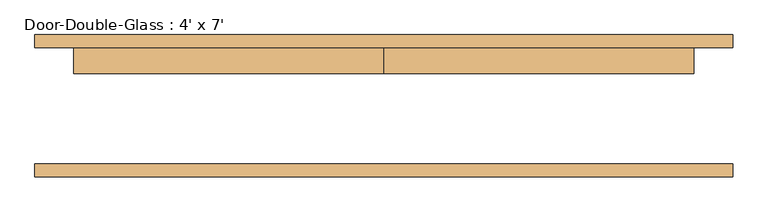
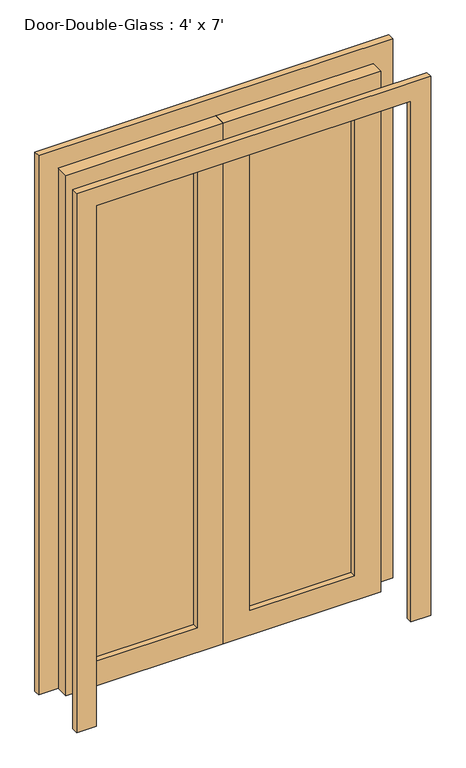
"""IFC4 building model written with IfcOpenShell, lengths in millimetres: door geometry, Door-Double-Glass : 4' x 7'."""

from ifc_helpers import new_model, si_unit, frame, origin, place, context, project, spatial, polyline, outline, extrude, source, transform, mapped, element, save


def door_double_glass_4_x_7_21e1f937(model_context):
    return source(origin(), model_context, "Body", "SweptSolid", [
        extrude(outline(polyline([(2133.6, 609.6), (2133.6, 0.0), (0.0, 0.0), (0.0, 609.6), (2133.6, 609.6)]), holes=[polyline([(2032.0, 508.0), (101.6, 508.0), (101.6, 101.6), (2032.0, 101.6), (2032.0, 508.0)])]), frame((0.0, 65.88125, 0.0), z_axis=(0.0, 1.0, 0.0), x_axis=(0.0, 0.0, 1.0)), (0.0, 0.0, 1.0), 50.8),
        extrude(outline(polyline([(2133.6, -609.6), (0.0, -609.6), (0.0, 0.0), (2133.6, 0.0), (2133.6, -609.6)]), holes=[polyline([(2032.0, -508.0), (2032.0, -101.6), (101.6, -101.6), (101.6, -508.0), (2032.0, -508.0)])]), frame((0.0, 65.88125, 0.0), z_axis=(0.0, 1.0, 0.0), x_axis=(0.0, 0.0, 1.0)), (0.0, 0.0, 1.0), 50.8),
        extrude(outline(polyline([(-508.0, 94.45625), (-101.6, 94.45625), (-101.6, 88.10625), (-508.0, 88.10625), (-508.0, 94.45625)])), frame((0.0, 0.0, 101.6), z_axis=(0.0, 0.0, 1.0), x_axis=(1.0, 0.0, 0.0)), (0.0, 0.0, 1.0), 1930.4),
        extrude(outline(polyline([(101.6, 94.45625), (508.0, 94.45625), (508.0, 88.10625), (101.6, 88.10625), (101.6, 94.45625)])), frame((0.0, 0.0, 101.6), z_axis=(0.0, 0.0, 1.0), x_axis=(1.0, 0.0, 0.0)), (0.0, 0.0, 1.0), 1930.4),
        extrude(outline(polyline([(0.0, 685.8), (2209.8, 685.8), (2209.8, -685.8), (0.0, -685.8), (0.0, -609.6), (2133.6, -609.6), (2133.6, 609.6), (0.0, 609.6), (0.0, 685.8)])), frame((0.0, -137.31875, 0.0), z_axis=(0.0, 1.0, 0.0), x_axis=(0.0, 0.0, 1.0)), (0.0, 0.0, 1.0), 25.4),
        extrude(outline(polyline([(0.0, 685.8), (2209.8, 685.8), (2209.8, -685.8), (0.0, -685.8), (0.0, -609.6), (2133.6, -609.6), (2133.6, 609.6), (0.0, 609.6), (0.0, 685.8)])), frame((0.0, 116.68125, 0.0), z_axis=(0.0, 1.0, 0.0), x_axis=(0.0, 0.0, 1.0)), (0.0, 0.0, 1.0), 25.4),
    ])


if __name__ == "__main__":
    model = new_model("IFC4")
    model_context = context("Model", 3, world=origin())
    ifc_project = project(units=[si_unit("LENGTHUNIT", "METRE", prefix="MILLI")], contexts=[model_context])
    site = spatial("IfcSite", under=ifc_project)
    building = spatial("IfcBuilding", under=site)
    placement = place(None, origin())
    door_double_glass_4_x_7_shape = door_double_glass_4_x_7_21e1f937(model_context)
    element("IfcDoor", 1, ObjectType="Door-Double-Glass : 4' x 7'", at=placement, inside=building, context=model_context, shape_type="MappedRepresentation", body=[
        mapped(door_double_glass_4_x_7_shape, transform((0.0, 0.0, 0.0), x_axis=(1.0, 0.0, 0.0), y_axis=(0.0, 1.0, 0.0), z_axis=(0.0, 0.0, 1.0))),
    ])
    save(model, "model.ifc")

# Revit data of these elements
# Type "Door-Double-Glass : 4' x 7'"
#   Type Mark = "16"
#   Construction Type Id = "opn-d45"
#   Assembly Code = "C1020"
#   Analytic Construction = "Wood frame, double glass door "
#   W = 2' - 0"
#   Thickness = 0' - 2"
#   Thermal Resistance (R) = 1.8150 (h·ft²·°F)/BTU
#   Swing Angle [instance default] = 90.00°
#   Heat Transfer Coefficient (U) = 0.5510 BTU/(h·ft²·°F)
#   Height = 7' - 0"
#   Bottom Rail = 0' - 4"
#   Top Rail = 0' - 4"
#   Stiles = 0' - 4"
#   Trim Projection = 0' - 1"
#   Trim Width = 0' - 3"
#   Width = 4' - 0"
#   Define Thermal Properties by = 1
#   Glazing = Glass
#   Panel Material = door black
#   Trim Material = Paint - Sienna
#   Visual Light Transmittance = 0
#   Solar Heat Gain Coefficient = 0
#   Function = (empty or 0)
#   Wall Closure = (empty or 0)
# Element 1 (IfcDoor, "Door-Double-Glass : 4' x 7'")
#   Materials on its faces: "door black", "Paint - Sienna", "Glass"
# Materials
#   "Glass": class "Glass", colour RGB 0 128 192, transparency 0.75, Description = "Soda Lime Glass", Cost = 0
#   "door black": class "Generic", colour RGB 120 120 120, transparency 0, Cost = 0
#   "Paint - Sienna": colour RGB 118 70 51, transparency 0, Cost = 0
